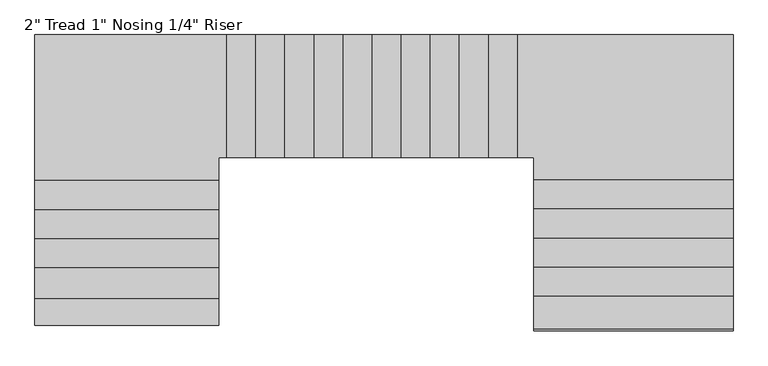
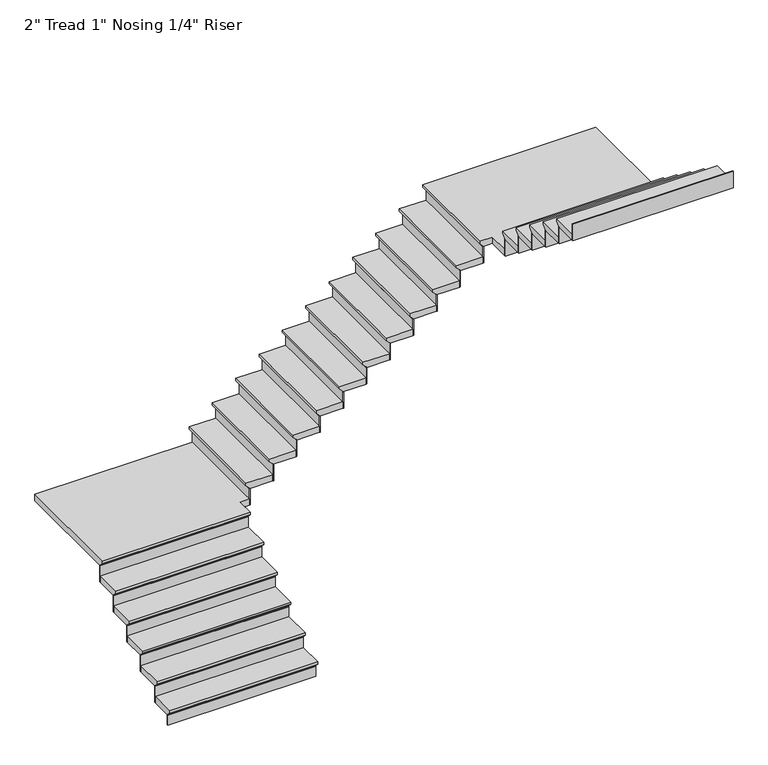
"""IFC4 building model written with IfcOpenShell, lengths in millimetres: stair flight geometry."""

from ifc_helpers import new_model, si_unit, origin, place, context, project, spatial, faceted_brep, source, transform, mapped, element, save


def stair_flight_92e1e4df(model_context):
    return source(origin(), model_context, "Body", "Brep", [
        faceted_brep([(-2368.6972892, 4718.9167606, 113.4717391), (-2368.6972892, 4718.9167606, 132.5217391), (-3493.0046642, 4718.9167606, 132.5217391), (-3493.0046642, 4718.9167606, 113.4717391), (-2368.6972892, 4744.3167606, 88.0717391), (-3493.0046642, 4744.3167606, 88.0717391), (-2368.6972892, 4909.4167606, 132.5217391), (-3493.0046642, 4909.4167606, 132.5217391), (-3493.0046642, 4744.3167606, 81.7217391), (-3493.0046642, 4909.4167606, 81.7217391), (-2368.6972892, 4909.4167606, 81.7217391), (-2368.6972892, 4744.3167606, 81.7217391)], [[[0, 1, 2, 3]], [[4, 0, 3, 5]], [[2, 1, 6, 7]], [[8, 9, 10, 11]], [[2, 7, 9, 8, 5, 3]], [[8, 11, 4, 5]], [[6, 1, 0, 4, 11, 10]], [[7, 6, 10, 9]]]),
        faceted_brep([(-2368.6972892, 4744.3167606, 81.7217391), (-2368.6972892, 4744.3167606, 0.0), (-2368.6972892, 4750.6667606, 0.0), (-2368.6972892, 4750.6667606, 81.7217391), (-3493.0046642, 4744.3167606, 81.7217391), (-3493.0046642, 4750.6667606, 81.7217391), (-3493.0046642, 4750.6667606, 0.0), (-3493.0046642, 4744.3167606, 0.0)], [[[0, 1, 2, 3]], [[4, 5, 6, 7]], [[1, 0, 4, 7]], [[2, 1, 7, 6]], [[3, 2, 6, 5]], [[0, 3, 5, 4]]]),
        faceted_brep([(-2368.6972892, 4909.4167606, 214.2434783), (-2368.6972892, 4909.4167606, 81.7217391), (-2368.6972892, 4915.7667606, 81.7217391), (-2368.6972892, 4915.7667606, 214.2434783), (-3493.0046642, 4909.4167606, 214.2434783), (-3493.0046642, 4915.7667606, 214.2434783), (-3493.0046642, 4915.7667606, 81.7217391), (-3493.0046642, 4909.4167606, 81.7217391)], [[[0, 1, 2, 3]], [[4, 5, 6, 7]], [[1, 0, 4, 7]], [[2, 1, 7, 6]], [[3, 2, 6, 5]], [[0, 3, 5, 4]]]),
        faceted_brep([(-3493.0046642, 4884.0167606, 265.0434783), (-2368.6972892, 4884.0167606, 265.0434783), (-2368.6972892, 5099.9164494, 265.0434783), (-3493.0046642, 5099.9164494, 265.0434783), (-3493.0046642, 4909.4167606, 214.2434783), (-3493.0046642, 5099.9164494, 214.2434783), (-2368.6972892, 5099.9164494, 214.2434783), (-2368.6972892, 4909.4167606, 214.2434783), (-3493.0046642, 4909.4167606, 220.5934783), (-3493.0046642, 4884.0167606, 245.9934783), (-2368.6972892, 4909.4167606, 220.5934783), (-2368.6972892, 4884.0167606, 245.9934783)], [[[0, 1, 2, 3]], [[4, 5, 6, 7]], [[0, 3, 5, 4, 8, 9]], [[4, 7, 10, 8]], [[2, 1, 11, 10, 7, 6]], [[3, 2, 6, 5]], [[11, 1, 0, 9]], [[10, 11, 9, 8]]]),
        faceted_brep([(-2368.6972892, 5099.9164494, 346.7652174), (-2368.6972892, 5099.9164494, 214.2434783), (-2368.6972892, 5106.2664494, 214.2434783), (-2368.6972892, 5106.2664494, 346.7652174), (-3493.0046642, 5099.9164494, 346.7652174), (-3493.0046642, 5106.2664494, 346.7652174), (-3493.0046642, 5106.2664494, 214.2434783), (-3493.0046642, 5099.9164494, 214.2434783)], [[[0, 1, 2, 3]], [[4, 5, 6, 7]], [[1, 0, 4, 7]], [[2, 1, 7, 6]], [[3, 2, 6, 5]], [[0, 3, 5, 4]]]),
        faceted_brep([(-3493.0046642, 5074.5164494, 397.5652174), (-2368.6972892, 5074.5164494, 397.5652174), (-2368.6972892, 5277.7164494, 397.5652174), (-3493.0046642, 5277.7164494, 397.5652174), (-3493.0046642, 5099.9164494, 346.7652174), (-3493.0046642, 5277.7164494, 346.7652174), (-2368.6972892, 5277.7164494, 346.7652174), (-2368.6972892, 5099.9164494, 346.7652174), (-3493.0046642, 5099.9164494, 353.1152174), (-3493.0046642, 5074.5164494, 378.5152174), (-2368.6972892, 5099.9164494, 353.1152174), (-2368.6972892, 5074.5164494, 378.5152174)], [[[0, 1, 2, 3]], [[4, 5, 6, 7]], [[0, 3, 5, 4, 8, 9]], [[4, 7, 10, 8]], [[2, 1, 11, 10, 7, 6]], [[3, 2, 6, 5]], [[11, 1, 0, 9]], [[10, 11, 9, 8]]]),
        faceted_brep([(-2368.6972892, 5277.7164494, 479.2869565), (-2368.6972892, 5277.7164494, 346.7652174), (-2368.6972892, 5284.0664494, 346.7652174), (-2368.6972892, 5284.0664494, 479.2869565), (-3493.0046642, 5277.7164494, 479.2869565), (-3493.0046642, 5284.0664494, 479.2869565), (-3493.0046642, 5284.0664494, 346.7652174), (-3493.0046642, 5277.7164494, 346.7652174)], [[[0, 1, 2, 3]], [[4, 5, 6, 7]], [[1, 0, 4, 7]], [[2, 1, 7, 6]], [[3, 2, 6, 5]], [[0, 3, 5, 4]]]),
        faceted_brep([(-3493.0046642, 5252.3164494, 530.0869565), (-2368.6972892, 5252.3164494, 530.0869565), (-2368.6972892, 5455.5164494, 530.0869565), (-3493.0046642, 5455.5164494, 530.0869565), (-3493.0046642, 5277.7164494, 479.2869565), (-3493.0046642, 5455.5164494, 479.2869565), (-2368.6972892, 5455.5164494, 479.2869565), (-2368.6972892, 5277.7164494, 479.2869565), (-3493.0046642, 5277.7164494, 485.6369565), (-3493.0046642, 5252.3164494, 511.0369565), (-2368.6972892, 5277.7164494, 485.6369565), (-2368.6972892, 5252.3164494, 511.0369565)], [[[0, 1, 2, 3]], [[4, 5, 6, 7]], [[0, 3, 5, 4, 8, 9]], [[4, 7, 10, 8]], [[2, 1, 11, 10, 7, 6]], [[3, 2, 6, 5]], [[11, 1, 0, 9]], [[10, 11, 9, 8]]]),
        faceted_brep([(-2368.6972892, 5455.5164494, 611.8086957), (-2368.6972892, 5455.5164494, 479.2869565), (-2368.6972892, 5461.8664494, 479.2869565), (-2368.6972892, 5461.8664494, 611.8086957), (-3493.0046642, 5455.5164494, 611.8086957), (-3493.0046642, 5461.8664494, 611.8086957), (-3493.0046642, 5461.8664494, 479.2869565), (-3493.0046642, 5455.5164494, 479.2869565)], [[[0, 1, 2, 3]], [[4, 5, 6, 7]], [[1, 0, 4, 7]], [[2, 1, 7, 6]], [[3, 2, 6, 5]], [[0, 3, 5, 4]]]),
        faceted_brep([(-3493.0046642, 5430.1164494, 662.6086957), (-2368.6972892, 5430.1164494, 662.6086957), (-2368.6972892, 5633.3167606, 662.6086957), (-3493.0046642, 5633.3167606, 662.6086957), (-3493.0046642, 5455.5164494, 611.8086957), (-3493.0046642, 5633.3167606, 611.8086957), (-2368.6972892, 5633.3167606, 611.8086957), (-2368.6972892, 5455.5164494, 611.8086957), (-3493.0046642, 5455.5164494, 618.1586957), (-3493.0046642, 5430.1164494, 643.5586957), (-2368.6972892, 5455.5164494, 618.1586957), (-2368.6972892, 5430.1164494, 643.5586957)], [[[0, 1, 2, 3]], [[4, 5, 6, 7]], [[0, 3, 5, 4, 8, 9]], [[4, 7, 10, 8]], [[2, 1, 11, 10, 7, 6]], [[3, 2, 6, 5]], [[11, 1, 0, 9]], [[10, 11, 9, 8]]]),
        faceted_brep([(-2368.6972892, 5633.3167606, 744.3304348), (-2368.6972892, 5633.3167606, 611.8086957), (-2368.6972892, 5639.6667606, 611.8086957), (-2368.6972892, 5639.6667606, 744.3304348), (-3493.0046642, 5633.3167606, 744.3304348), (-3493.0046642, 5639.6667606, 744.3304348), (-3493.0046642, 5639.6667606, 611.8086957), (-3493.0046642, 5633.3167606, 611.8086957)], [[[0, 1, 2, 3]], [[4, 5, 6, 7]], [[1, 0, 4, 7]], [[2, 1, 7, 6]], [[3, 2, 6, 5]], [[0, 3, 5, 4]]]),
        faceted_brep([(-2295.032382, 6496.9167606, 795.1304348), (-3493.0046642, 6496.9167606, 795.1304348), (-3493.0046642, 5607.9167606, 795.1304348), (-2368.6972892, 5607.9167606, 795.1304348), (-2368.6972892, 5746.5536537, 795.1304348), (-2295.032382, 5746.5536537, 795.1304348), (-3493.0046642, 6496.9167606, 744.3304348), (-2295.032382, 6496.9167606, 744.3304348), (-2295.032382, 5746.5536537, 744.3304348), (-2368.6972892, 5746.5536537, 744.3304348), (-2368.6972892, 5633.3167606, 744.3304348), (-3493.0046642, 5633.3167606, 744.3304348), (-3493.0046642, 5633.3167606, 750.6804348), (-3493.0046642, 5607.9167606, 776.0804348), (-2368.6972892, 5633.3167606, 750.6804348), (-2368.6972892, 5607.9167606, 776.0804348)], [[[0, 1, 2, 3, 4, 5]], [[6, 7, 8, 9, 10, 11]], [[1, 0, 7, 6]], [[2, 1, 6, 11, 12, 13]], [[11, 10, 14, 12]], [[4, 3, 15, 14, 10, 9]], [[5, 4, 9, 8]], [[0, 5, 8, 7]], [[15, 3, 2, 13]], [[14, 15, 13, 12]]]),
        faceted_brep([(-2295.032382, 5746.5536537, 876.8521739), (-2295.032382, 5746.5536537, 744.3304348), (-2288.682382, 5746.5536537, 744.3304348), (-2288.682382, 5746.5536537, 876.8521739), (-2295.032382, 6496.9167606, 876.8521739), (-2288.682382, 6496.9167606, 876.8521739), (-2288.682382, 6496.9167606, 744.3304348), (-2295.032382, 6496.9167606, 744.3304348)], [[[0, 1, 2, 3]], [[4, 5, 6, 7]], [[1, 0, 4, 7]], [[2, 1, 7, 6]], [[3, 2, 6, 5]], [[0, 3, 5, 4]]]),
        faceted_brep([(-2320.432382, 6496.9167606, 927.6521739), (-2320.432382, 5746.5536537, 927.6521739), (-2117.232382, 5746.5536537, 927.6521739), (-2117.232382, 6496.9167606, 927.6521739), (-2295.032382, 6496.9167606, 876.8521739), (-2117.232382, 6496.9167606, 876.8521739), (-2117.232382, 5746.5536537, 876.8521739), (-2295.032382, 5746.5536537, 876.8521739), (-2295.032382, 6496.9167606, 883.2021739), (-2320.432382, 6496.9167606, 908.6021739), (-2295.032382, 5746.5536537, 883.2021739), (-2320.432382, 5746.5536537, 908.6021739)], [[[0, 1, 2, 3]], [[4, 5, 6, 7]], [[0, 3, 5, 4, 8, 9]], [[4, 7, 10, 8]], [[2, 1, 11, 10, 7, 6]], [[3, 2, 6, 5]], [[11, 1, 0, 9]], [[10, 11, 9, 8]]]),
        faceted_brep([(-2117.232382, 5746.5536537, 1009.373913), (-2117.232382, 5746.5536537, 876.8521739), (-2110.882382, 5746.5536537, 876.8521739), (-2110.882382, 5746.5536537, 1009.373913), (-2117.232382, 6496.9167606, 1009.373913), (-2110.882382, 6496.9167606, 1009.373913), (-2110.882382, 6496.9167606, 876.8521739), (-2117.232382, 6496.9167606, 876.8521739)], [[[0, 1, 2, 3]], [[4, 5, 6, 7]], [[1, 0, 4, 7]], [[2, 1, 7, 6]], [[3, 2, 6, 5]], [[0, 3, 5, 4]]]),
        faceted_brep([(-2142.632382, 6496.9167606, 1060.173913), (-2142.632382, 5746.5536537, 1060.173913), (-1939.432382, 5746.5536537, 1060.173913), (-1939.432382, 6496.9167606, 1060.173913), (-2117.232382, 6496.9167606, 1009.373913), (-1939.432382, 6496.9167606, 1009.373913), (-1939.432382, 5746.5536537, 1009.373913), (-2117.232382, 5746.5536537, 1009.373913), (-2117.232382, 6496.9167606, 1015.723913), (-2142.632382, 6496.9167606, 1041.123913), (-2117.232382, 5746.5536537, 1015.723913), (-2142.632382, 5746.5536537, 1041.123913)], [[[0, 1, 2, 3]], [[4, 5, 6, 7]], [[0, 3, 5, 4, 8, 9]], [[4, 7, 10, 8]], [[2, 1, 11, 10, 7, 6]], [[3, 2, 6, 5]], [[11, 1, 0, 9]], [[10, 11, 9, 8]]]),
        faceted_brep([(-1939.432382, 5746.5536537, 1141.8956522), (-1939.432382, 5746.5536537, 1009.373913), (-1933.082382, 5746.5536537, 1009.373913), (-1933.082382, 5746.5536537, 1141.8956522), (-1939.432382, 6496.9167606, 1141.8956522), (-1933.082382, 6496.9167606, 1141.8956522), (-1933.082382, 6496.9167606, 1009.373913), (-1939.432382, 6496.9167606, 1009.373913)], [[[0, 1, 2, 3]], [[4, 5, 6, 7]], [[1, 0, 4, 7]], [[2, 1, 7, 6]], [[3, 2, 6, 5]], [[0, 3, 5, 4]]]),
        faceted_brep([(-1964.832382, 6496.9167606, 1192.6956522), (-1964.832382, 5746.5536537, 1192.6956522), (-1761.632382, 5746.5536537, 1192.6956522), (-1761.632382, 6496.9167606, 1192.6956522), (-1939.432382, 6496.9167606, 1141.8956522), (-1761.632382, 6496.9167606, 1141.8956522), (-1761.632382, 5746.5536537, 1141.8956522), (-1939.432382, 5746.5536537, 1141.8956522), (-1939.432382, 6496.9167606, 1148.2456522), (-1964.832382, 6496.9167606, 1173.6456522), (-1939.432382, 5746.5536537, 1148.2456522), (-1964.832382, 5746.5536537, 1173.6456522)], [[[0, 1, 2, 3]], [[4, 5, 6, 7]], [[0, 3, 5, 4, 8, 9]], [[4, 7, 10, 8]], [[2, 1, 11, 10, 7, 6]], [[3, 2, 6, 5]], [[11, 1, 0, 9]], [[10, 11, 9, 8]]]),
        faceted_brep([(-1761.632382, 5746.5536537, 1274.4173913), (-1761.632382, 5746.5536537, 1141.8956522), (-1755.282382, 5746.5536537, 1141.8956522), (-1755.282382, 5746.5536537, 1274.4173913), (-1761.632382, 6496.9167606, 1274.4173913), (-1755.282382, 6496.9167606, 1274.4173913), (-1755.282382, 6496.9167606, 1141.8956522), (-1761.632382, 6496.9167606, 1141.8956522)], [[[0, 1, 2, 3]], [[4, 5, 6, 7]], [[1, 0, 4, 7]], [[2, 1, 7, 6]], [[3, 2, 6, 5]], [[0, 3, 5, 4]]]),
        faceted_brep([(-1787.032382, 6496.9167606, 1325.2173913), (-1787.032382, 5746.5536537, 1325.2173913), (-1583.832382, 5746.5536537, 1325.2173913), (-1583.832382, 6496.9167606, 1325.2173913), (-1761.632382, 6496.9167606, 1274.4173913), (-1583.832382, 6496.9167606, 1274.4173913), (-1583.832382, 5746.5536537, 1274.4173913), (-1761.632382, 5746.5536537, 1274.4173913), (-1761.632382, 6496.9167606, 1280.7673913), (-1787.032382, 6496.9167606, 1306.1673913), (-1761.632382, 5746.5536537, 1280.7673913), (-1787.032382, 5746.5536537, 1306.1673913)], [[[0, 1, 2, 3]], [[4, 5, 6, 7]], [[0, 3, 5, 4, 8, 9]], [[4, 7, 10, 8]], [[2, 1, 11, 10, 7, 6]], [[3, 2, 6, 5]], [[11, 1, 0, 9]], [[10, 11, 9, 8]]]),
        faceted_brep([(-1583.832382, 5746.5536537, 1406.9391304), (-1583.832382, 5746.5536537, 1274.4173913), (-1577.482382, 5746.5536537, 1274.4173913), (-1577.482382, 5746.5536537, 1406.9391304), (-1583.832382, 6496.9167606, 1406.9391304), (-1577.482382, 6496.9167606, 1406.9391304), (-1577.482382, 6496.9167606, 1274.4173913), (-1583.832382, 6496.9167606, 1274.4173913)], [[[0, 1, 2, 3]], [[4, 5, 6, 7]], [[1, 0, 4, 7]], [[2, 1, 7, 6]], [[3, 2, 6, 5]], [[0, 3, 5, 4]]]),
        faceted_brep([(-1609.232382, 6496.9167606, 1457.7391304), (-1609.232382, 5746.5536537, 1457.7391304), (-1406.032382, 5746.5536537, 1457.7391304), (-1406.032382, 6496.9167606, 1457.7391304), (-1583.832382, 6496.9167606, 1406.9391304), (-1406.032382, 6496.9167606, 1406.9391304), (-1406.032382, 5746.5536537, 1406.9391304), (-1583.832382, 5746.5536537, 1406.9391304), (-1583.832382, 6496.9167606, 1413.2891304), (-1609.232382, 6496.9167606, 1438.6891304), (-1583.832382, 5746.5536537, 1413.2891304), (-1609.232382, 5746.5536537, 1438.6891304)], [[[0, 1, 2, 3]], [[4, 5, 6, 7]], [[0, 3, 5, 4, 8, 9]], [[4, 7, 10, 8]], [[2, 1, 11, 10, 7, 6]], [[3, 2, 6, 5]], [[11, 1, 0, 9]], [[10, 11, 9, 8]]]),
        faceted_brep([(-1406.032382, 5746.5536537, 1539.4608696), (-1406.032382, 5746.5536537, 1406.9391304), (-1399.682382, 5746.5536537, 1406.9391304), (-1399.682382, 5746.5536537, 1539.4608696), (-1406.032382, 6496.9167606, 1539.4608696), (-1399.682382, 6496.9167606, 1539.4608696), (-1399.682382, 6496.9167606, 1406.9391304), (-1406.032382, 6496.9167606, 1406.9391304)], [[[0, 1, 2, 3]], [[4, 5, 6, 7]], [[1, 0, 4, 7]], [[2, 1, 7, 6]], [[3, 2, 6, 5]], [[0, 3, 5, 4]]]),
        faceted_brep([(-1431.432382, 6496.9167606, 1590.2608696), (-1431.432382, 5746.5536537, 1590.2608696), (-1228.232382, 5746.5536537, 1590.2608696), (-1228.232382, 6496.9167606, 1590.2608696), (-1406.032382, 6496.9167606, 1539.4608696), (-1228.232382, 6496.9167606, 1539.4608696), (-1228.232382, 5746.5536537, 1539.4608696), (-1406.032382, 5746.5536537, 1539.4608696), (-1406.032382, 6496.9167606, 1545.8108696), (-1431.432382, 6496.9167606, 1571.2108696), (-1406.032382, 5746.5536537, 1545.8108696), (-1431.432382, 5746.5536537, 1571.2108696)], [[[0, 1, 2, 3]], [[4, 5, 6, 7]], [[0, 3, 5, 4, 8, 9]], [[4, 7, 10, 8]], [[2, 1, 11, 10, 7, 6]], [[3, 2, 6, 5]], [[11, 1, 0, 9]], [[10, 11, 9, 8]]]),
        faceted_brep([(-1228.232382, 5746.5536537, 1671.9826087), (-1228.232382, 5746.5536537, 1539.4608696), (-1221.882382, 5746.5536537, 1539.4608696), (-1221.882382, 5746.5536537, 1671.9826087), (-1228.232382, 6496.9167606, 1671.9826087), (-1221.882382, 6496.9167606, 1671.9826087), (-1221.882382, 6496.9167606, 1539.4608696), (-1228.232382, 6496.9167606, 1539.4608696)], [[[0, 1, 2, 3]], [[4, 5, 6, 7]], [[1, 0, 4, 7]], [[2, 1, 7, 6]], [[3, 2, 6, 5]], [[0, 3, 5, 4]]]),
        faceted_brep([(-1253.632382, 6496.9167606, 1722.7826087), (-1253.632382, 5746.5536537, 1722.7826087), (-1050.432382, 5746.5536537, 1722.7826087), (-1050.432382, 6496.9167606, 1722.7826087), (-1228.232382, 6496.9167606, 1671.9826087), (-1050.432382, 6496.9167606, 1671.9826087), (-1050.432382, 5746.5536537, 1671.9826087), (-1228.232382, 5746.5536537, 1671.9826087), (-1228.232382, 6496.9167606, 1678.3326087), (-1253.632382, 6496.9167606, 1703.7326087), (-1228.232382, 5746.5536537, 1678.3326087), (-1253.632382, 5746.5536537, 1703.7326087)], [[[0, 1, 2, 3]], [[4, 5, 6, 7]], [[0, 3, 5, 4, 8, 9]], [[4, 7, 10, 8]], [[2, 1, 11, 10, 7, 6]], [[3, 2, 6, 5]], [[11, 1, 0, 9]], [[10, 11, 9, 8]]]),
        faceted_brep([(-1050.432382, 5746.5536537, 1804.5043478), (-1050.432382, 5746.5536537, 1671.9826087), (-1044.082382, 5746.5536537, 1671.9826087), (-1044.082382, 5746.5536537, 1804.5043478), (-1050.432382, 6496.9167606, 1804.5043478), (-1044.082382, 6496.9167606, 1804.5043478), (-1044.082382, 6496.9167606, 1671.9826087), (-1050.432382, 6496.9167606, 1671.9826087)], [[[0, 1, 2, 3]], [[4, 5, 6, 7]], [[1, 0, 4, 7]], [[2, 1, 7, 6]], [[3, 2, 6, 5]], [[0, 3, 5, 4]]]),
        faceted_brep([(-1075.832382, 6496.9167606, 1855.3043478), (-1075.832382, 5746.5536537, 1855.3043478), (-872.632382, 5746.5536537, 1855.3043478), (-872.632382, 6496.9167606, 1855.3043478), (-1050.432382, 6496.9167606, 1804.5043478), (-872.632382, 6496.9167606, 1804.5043478), (-872.632382, 5746.5536537, 1804.5043478), (-1050.432382, 5746.5536537, 1804.5043478), (-1050.432382, 6496.9167606, 1810.8543478), (-1075.832382, 6496.9167606, 1836.2543478), (-1050.432382, 5746.5536537, 1810.8543478), (-1075.832382, 5746.5536537, 1836.2543478)], [[[0, 1, 2, 3]], [[4, 5, 6, 7]], [[0, 3, 5, 4, 8, 9]], [[4, 7, 10, 8]], [[2, 1, 11, 10, 7, 6]], [[3, 2, 6, 5]], [[11, 1, 0, 9]], [[10, 11, 9, 8]]]),
        faceted_brep([(-872.632382, 5746.5536537, 1937.026087), (-872.632382, 5746.5536537, 1804.5043478), (-866.282382, 5746.5536537, 1804.5043478), (-866.282382, 5746.5536537, 1937.026087), (-872.632382, 6496.9167606, 1937.026087), (-866.282382, 6496.9167606, 1937.026087), (-866.282382, 6496.9167606, 1804.5043478), (-872.632382, 6496.9167606, 1804.5043478)], [[[0, 1, 2, 3]], [[4, 5, 6, 7]], [[1, 0, 4, 7]], [[2, 1, 7, 6]], [[3, 2, 6, 5]], [[0, 3, 5, 4]]]),
        faceted_brep([(-898.032382, 6496.9167606, 1987.826087), (-898.032382, 5746.5536537, 1987.826087), (-694.832382, 5746.5536537, 1987.826087), (-694.832382, 6496.9167606, 1987.826087), (-872.632382, 6496.9167606, 1937.026087), (-694.832382, 6496.9167606, 1937.026087), (-694.832382, 5746.5536537, 1937.026087), (-872.632382, 5746.5536537, 1937.026087), (-872.632382, 6496.9167606, 1943.376087), (-898.032382, 6496.9167606, 1968.776087), (-872.632382, 5746.5536537, 1943.376087), (-898.032382, 5746.5536537, 1968.776087)], [[[0, 1, 2, 3]], [[4, 5, 6, 7]], [[0, 3, 5, 4, 8, 9]], [[4, 7, 10, 8]], [[2, 1, 11, 10, 7, 6]], [[3, 2, 6, 5]], [[11, 1, 0, 9]], [[10, 11, 9, 8]]]),
        faceted_brep([(-694.832382, 5746.5536537, 2069.5478261), (-694.832382, 5746.5536537, 1937.026087), (-688.482382, 5746.5536537, 1937.026087), (-688.482382, 5746.5536537, 2069.5478261), (-694.832382, 6496.9167606, 2069.5478261), (-688.482382, 6496.9167606, 2069.5478261), (-688.482382, 6496.9167606, 1937.026087), (-694.832382, 6496.9167606, 1937.026087)], [[[0, 1, 2, 3]], [[4, 5, 6, 7]], [[1, 0, 4, 7]], [[2, 1, 7, 6]], [[3, 2, 6, 5]], [[0, 3, 5, 4]]]),
        faceted_brep([(-720.232382, 6496.9167606, 2120.3478261), (-720.232382, 5746.5536537, 2120.3478261), (-517.032382, 5746.5536537, 2120.3478261), (-517.032382, 6496.9167606, 2120.3478261), (-694.832382, 6496.9167606, 2069.5478261), (-517.032382, 6496.9167606, 2069.5478261), (-517.032382, 5746.5536537, 2069.5478261), (-694.832382, 5746.5536537, 2069.5478261), (-694.832382, 6496.9167606, 2075.8978261), (-720.232382, 6496.9167606, 2101.2978261), (-694.832382, 5746.5536537, 2075.8978261), (-720.232382, 5746.5536537, 2101.2978261)], [[[0, 1, 2, 3]], [[4, 5, 6, 7]], [[0, 3, 5, 4, 8, 9]], [[4, 7, 10, 8]], [[2, 1, 11, 10, 7, 6]], [[3, 2, 6, 5]], [[11, 1, 0, 9]], [[10, 11, 9, 8]]]),
        faceted_brep([(-517.032382, 5746.5536537, 2202.0695652), (-517.032382, 5746.5536537, 2069.5478261), (-510.682382, 5746.5536537, 2069.5478261), (-510.682382, 5746.5536537, 2202.0695652), (-517.032382, 6496.9167606, 2202.0695652), (-510.682382, 6496.9167606, 2202.0695652), (-510.682382, 6496.9167606, 2069.5478261), (-517.032382, 6496.9167606, 2069.5478261)], [[[0, 1, 2, 3]], [[4, 5, 6, 7]], [[1, 0, 4, 7]], [[2, 1, 7, 6]], [[3, 2, 6, 5]], [[0, 3, 5, 4]]]),
        faceted_brep([(774.1953358, 5582.5167606, 2252.8695652), (774.1953358, 6496.9167606, 2252.8695652), (-542.432382, 6496.9167606, 2252.8695652), (-542.432382, 5746.5536537, 2252.8695652), (-445.0046642, 5746.5536537, 2252.8695652), (-445.0046642, 5582.5167606, 2252.8695652), (774.1953358, 6496.9167606, 2202.0695652), (774.1953358, 5582.5167606, 2202.0695652), (-445.0046642, 5582.5167606, 2202.0695652), (-445.0046642, 5746.5536537, 2202.0695652), (-517.032382, 5746.5536537, 2202.0695652), (-517.032382, 6496.9167606, 2202.0695652), (-517.032382, 6496.9167606, 2208.4195652), (-542.432382, 6496.9167606, 2233.8195652), (-517.032382, 5746.5536537, 2208.4195652), (-542.432382, 5746.5536537, 2233.8195652)], [[[0, 1, 2, 3, 4, 5]], [[6, 7, 8, 9, 10, 11]], [[1, 0, 7, 6]], [[2, 1, 6, 11, 12, 13]], [[11, 10, 14, 12]], [[4, 3, 15, 14, 10, 9]], [[5, 4, 9, 8]], [[0, 5, 8, 7]], [[15, 3, 2, 13]], [[14, 15, 13, 12]]]),
        faceted_brep([(-445.0046642, 5582.5167606, 2334.5913043), (-445.0046642, 5582.5167606, 2202.0695652), (-445.0046642, 5576.1667606, 2202.0695652), (-445.0046642, 5576.1667606, 2334.5913043), (774.1953358, 5582.5167606, 2334.5913043), (774.1953358, 5576.1667606, 2334.5913043), (774.1953358, 5576.1667606, 2202.0695652), (774.1953358, 5582.5167606, 2202.0695652)], [[[0, 1, 2, 3]], [[4, 5, 6, 7]], [[1, 0, 4, 7]], [[2, 1, 7, 6]], [[3, 2, 6, 5]], [[0, 3, 5, 4]]]),
        faceted_brep([(774.1953358, 5607.9167606, 2385.3913043), (-445.0046642, 5607.9167606, 2385.3913043), (-445.0046642, 5404.7164494, 2385.3913043), (774.1953358, 5404.7164494, 2385.3913043), (774.1953358, 5582.5167606, 2334.5913043), (774.1953358, 5404.7164494, 2334.5913043), (-445.0046642, 5404.7164494, 2334.5913043), (-445.0046642, 5582.5167606, 2334.5913043), (774.1953358, 5582.5167606, 2340.9413043), (774.1953358, 5607.9167606, 2366.3413043), (-445.0046642, 5582.5167606, 2340.9413043), (-445.0046642, 5607.9167606, 2366.3413043)], [[[0, 1, 2, 3]], [[4, 5, 6, 7]], [[0, 3, 5, 4, 8, 9]], [[4, 7, 10, 8]], [[2, 1, 11, 10, 7, 6]], [[3, 2, 6, 5]], [[11, 1, 0, 9]], [[10, 11, 9, 8]]]),
        faceted_brep([(-445.0046642, 5404.7164494, 2467.1130435), (-445.0046642, 5404.7164494, 2334.5913043), (-445.0046642, 5398.3664494, 2334.5913043), (-445.0046642, 5398.3664494, 2467.1130435), (774.1953358, 5404.7164494, 2467.1130435), (774.1953358, 5398.3664494, 2467.1130435), (774.1953358, 5398.3664494, 2334.5913043), (774.1953358, 5404.7164494, 2334.5913043)], [[[0, 1, 2, 3]], [[4, 5, 6, 7]], [[1, 0, 4, 7]], [[2, 1, 7, 6]], [[3, 2, 6, 5]], [[0, 3, 5, 4]]]),
        faceted_brep([(774.1953358, 5430.1164494, 2517.9130435), (-445.0046642, 5430.1164494, 2517.9130435), (-445.0046642, 5226.9164494, 2517.9130435), (774.1953358, 5226.9164494, 2517.9130435), (774.1953358, 5404.7164494, 2467.1130435), (774.1953358, 5226.9164494, 2467.1130435), (-445.0046642, 5226.9164494, 2467.1130435), (-445.0046642, 5404.7164494, 2467.1130435), (774.1953358, 5404.7164494, 2473.4630435), (774.1953358, 5430.1164494, 2498.8630435), (-445.0046642, 5404.7164494, 2473.4630435), (-445.0046642, 5430.1164494, 2498.8630435)], [[[0, 1, 2, 3]], [[4, 5, 6, 7]], [[0, 3, 5, 4, 8, 9]], [[4, 7, 10, 8]], [[2, 1, 11, 10, 7, 6]], [[3, 2, 6, 5]], [[11, 1, 0, 9]], [[10, 11, 9, 8]]]),
        faceted_brep([(-445.0046642, 5226.9164494, 2599.6347826), (-445.0046642, 5226.9164494, 2467.1130435), (-445.0046642, 5220.5664494, 2467.1130435), (-445.0046642, 5220.5664494, 2599.6347826), (774.1953358, 5226.9164494, 2599.6347826), (774.1953358, 5220.5664494, 2599.6347826), (774.1953358, 5220.5664494, 2467.1130435), (774.1953358, 5226.9164494, 2467.1130435)], [[[0, 1, 2, 3]], [[4, 5, 6, 7]], [[1, 0, 4, 7]], [[2, 1, 7, 6]], [[3, 2, 6, 5]], [[0, 3, 5, 4]]]),
        faceted_brep([(774.1953358, 5252.3164494, 2650.4347826), (-445.0046642, 5252.3164494, 2650.4347826), (-445.0046642, 5049.1164494, 2650.4347826), (774.1953358, 5049.1164494, 2650.4347826), (774.1953358, 5226.9164494, 2599.6347826), (774.1953358, 5049.1164494, 2599.6347826), (-445.0046642, 5049.1164494, 2599.6347826), (-445.0046642, 5226.9164494, 2599.6347826), (774.1953358, 5226.9164494, 2605.9847826), (774.1953358, 5252.3164494, 2631.3847826), (-445.0046642, 5226.9164494, 2605.9847826), (-445.0046642, 5252.3164494, 2631.3847826)], [[[0, 1, 2, 3]], [[4, 5, 6, 7]], [[0, 3, 5, 4, 8, 9]], [[4, 7, 10, 8]], [[2, 1, 11, 10, 7, 6]], [[3, 2, 6, 5]], [[11, 1, 0, 9]], [[10, 11, 9, 8]]]),
        faceted_brep([(-445.0046642, 5049.1164494, 2732.1565217), (-445.0046642, 5049.1164494, 2599.6347826), (-445.0046642, 5042.7664494, 2599.6347826), (-445.0046642, 5042.7664494, 2732.1565217), (774.1953358, 5049.1164494, 2732.1565217), (774.1953358, 5042.7664494, 2732.1565217), (774.1953358, 5042.7664494, 2599.6347826), (774.1953358, 5049.1164494, 2599.6347826)], [[[0, 1, 2, 3]], [[4, 5, 6, 7]], [[1, 0, 4, 7]], [[2, 1, 7, 6]], [[3, 2, 6, 5]], [[0, 3, 5, 4]]]),
        faceted_brep([(774.1953358, 5074.5164494, 2782.9565217), (-445.0046642, 5074.5164494, 2782.9565217), (-445.0046642, 4871.3164494, 2782.9565217), (774.1953358, 4871.3164494, 2782.9565217), (774.1953358, 5049.1164494, 2732.1565217), (774.1953358, 4871.3164494, 2732.1565217), (-445.0046642, 4871.3164494, 2732.1565217), (-445.0046642, 5049.1164494, 2732.1565217), (774.1953358, 5049.1164494, 2738.5065217), (774.1953358, 5074.5164494, 2763.9065217), (-445.0046642, 5049.1164494, 2738.5065217), (-445.0046642, 5074.5164494, 2763.9065217)], [[[0, 1, 2, 3]], [[4, 5, 6, 7]], [[0, 3, 5, 4, 8, 9]], [[4, 7, 10, 8]], [[2, 1, 11, 10, 7, 6]], [[3, 2, 6, 5]], [[11, 1, 0, 9]], [[10, 11, 9, 8]]]),
        faceted_brep([(-445.0046642, 4871.3164494, 2864.6782609), (-445.0046642, 4871.3164494, 2732.1565217), (-445.0046642, 4864.9664494, 2732.1565217), (-445.0046642, 4864.9664494, 2864.6782609), (774.1953358, 4871.3164494, 2864.6782609), (774.1953358, 4864.9664494, 2864.6782609), (774.1953358, 4864.9664494, 2732.1565217), (774.1953358, 4871.3164494, 2732.1565217)], [[[0, 1, 2, 3]], [[4, 5, 6, 7]], [[1, 0, 4, 7]], [[2, 1, 7, 6]], [[3, 2, 6, 5]], [[0, 3, 5, 4]]]),
        faceted_brep([(-445.0046642, 4693.5167606, 2997.2), (-445.0046642, 4693.5167606, 2864.6782609), (-445.0046642, 4687.1667606, 2864.6782609), (-445.0046642, 4687.1667606, 2997.2), (774.1953358, 4693.5167606, 2997.2), (774.1953358, 4687.1667606, 2997.2), (774.1953358, 4687.1667606, 2864.6782609), (774.1953358, 4693.5167606, 2864.6782609)], [[[0, 1, 2, 3]], [[4, 5, 6, 7]], [[1, 0, 4, 7]], [[2, 1, 7, 6]], [[3, 2, 6, 5]], [[0, 3, 5, 4]]]),
        faceted_brep([(774.1953358, 4896.7164494, 2915.4782609), (-445.0046642, 4896.7164494, 2915.4782609), (-445.0046642, 4693.5167606, 2915.4782609), (774.1953358, 4693.5167606, 2915.4782609), (774.1953358, 4871.3164494, 2864.6782609), (774.1953358, 4693.5167606, 2864.6782609), (-445.0046642, 4693.5167606, 2864.6782609), (-445.0046642, 4871.3164494, 2864.6782609), (774.1953358, 4871.3164494, 2871.0282609), (774.1953358, 4896.7164494, 2896.4282609), (-445.0046642, 4871.3164494, 2871.0282609), (-445.0046642, 4896.7164494, 2896.4282609)], [[[0, 1, 2, 3]], [[4, 5, 6, 7]], [[0, 3, 5, 4, 8, 9]], [[4, 7, 10, 8]], [[2, 1, 11, 10, 7, 6]], [[3, 2, 6, 5]], [[11, 1, 0, 9]], [[10, 11, 9, 8]]]),
    ])


if __name__ == "__main__":
    model = new_model("IFC4")
    model_context = context("Model", 3, world=origin())
    ifc_project = project(units=[si_unit("LENGTHUNIT", "METRE", prefix="MILLI")], contexts=[model_context])
    site = spatial("IfcSite", under=ifc_project)
    building = spatial("IfcBuilding", under=site)
    placement = place(None, origin())
    stair_flight_shape = stair_flight_92e1e4df(model_context)
    element("IfcStairFlight", 1, ObjectType="2\" Tread 1\" Nosing 1/4\" Riser", at=placement, inside=building, context=model_context, shape_type="MappedRepresentation", body=[
        mapped(stair_flight_shape, transform((0.0, 0.0, 0.0), x_axis=(1.0, 0.0, 0.0), y_axis=(0.0, 1.0, 0.0), z_axis=(0.0, 0.0, 1.0))),
    ])
    save(model, "model.ifc")
